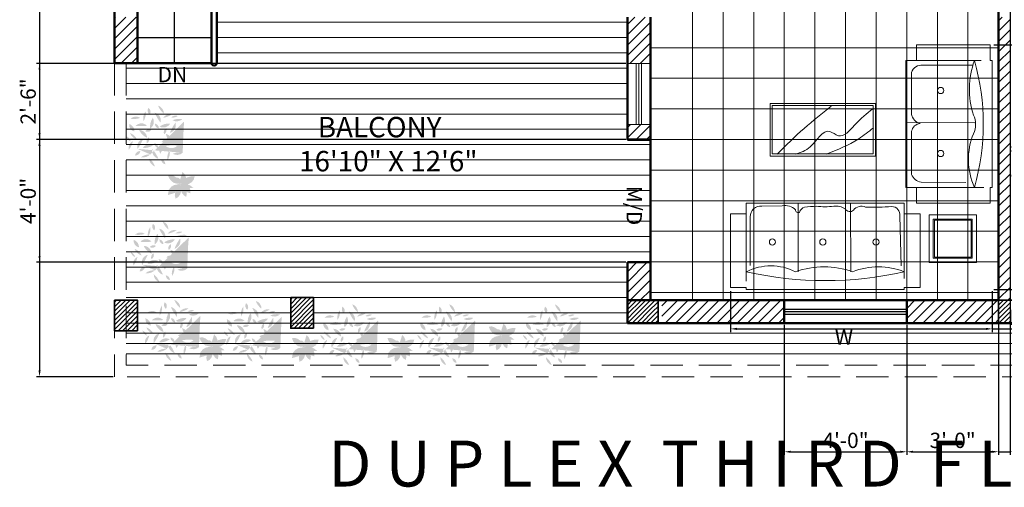
# Model space of a CAD drawing. Units: millimetres. Extents: x 225995 to 227247, y 225507 to 226008.
# Tile 11 of 23: x 226643 to 227029, y 225507 to 225691. Entities that reach past the tile are written whole.
import ezdxf

# ---------------------------------------------------------------- set-up
doc = ezdxf.new("R2010")
doc.units = ezdxf.units.MM
doc.linetypes.add('DASHED', pattern=[19.049999999999997, 12.7, -6.349999999999999])
for name, color, linetype, lineweight in [('A-ANNO-DIMS', 2, 'Continuous', 18), ('A-ANNO-TEXT', 3, 'Continuous', 18), ('A-AREA-IDEN', 30, 'Continuous', 18), ('A-COLS', 40, 'Continuous', 35), ('A-FLOR-PATT', 8, 'Continuous', 13), ('A-FLOR-STRS', 141, 'Continuous', 25), ('A-FURN', 9, 'Continuous', 18), ('A-GLAZ', 4, 'Continuous', 25), ('A-WALL', 7, 'Continuous', 50), ('A-WALL-OVHD', 1, 'DASHED', 18), ('A-WALL-PATT', 8, 'Continuous', 13)]:
    doc.layers.add(name, color=color, linetype=linetype, lineweight=lineweight)
doc.styles.get("Standard").update_dxf_attribs({"font": 'arial.ttf'})
doc.dimstyles.new('ISO-25', dxfattribs={"dimtxt": 6, "dimasz": 2.5, "dimexe": 1.25, "dimexo": 0.625, "dimtad": 1, "dimdec": 0, "dimlunit": 3, "dimtxsty": 'Standard', "dimcen": 2.5, "dimadec": 0, "dimazin": 0, "dimtfac": 1, "dimtdec": 0, "dimtmove": 0, "dimatfit": 3, "dimfxl": 1, "dimarcsym": 0})
pattern_1 = [(45, (646.0462645871739, 0.9310331261949613), (-2.020557627240559, 2.020557627240559), [])]
pattern_2 = [(45, (646.0462645871739, -119.068966873805), (-0.8980256121069157, 0.8980256121069157), [])]
pattern_3 = [(45, (500.5462645871448, -119.0689668737759), (-0.8980256121069157, 0.8980256121069157), [])]
pattern_4 = [(45, (0, 0), (-2.020557627240559, 2.020557627240559), [])]

# ---------------------------------------------------------------- blocks, each defined once
blk = doc.blocks.new('A$C412119AE')
for p, q in [((1765.943953579699, 2175.983816529711), (1765.943953579699, 2325.983816529712)), ((1765.943953579699, 2325.983816529712), (2465.943953579699, 2325.983816529712)), ((2465.943953579699, 2325.983816529712), (2465.943953579699, 2175.983816529711)), ((1665.943953579699, 2175.983816529711), (1765.943953579699, 2175.983816529711)), ((1665.943953579699, 2175.983816529711), (1665.943953579699, 970.8113427770732)), ((2379.086550219509, 2175.983816529711), (1665.943953579699, 2175.983816529711)), ((2465.943953579699, 2175.983816529711), (2485.943953579699, 2175.983816529711)), ((2485.943953579699, 2175.983816529711), (2485.943953579699, 970.8113427770732)), ((1719.402132396004, 1668.149708631943), (1719.402132396004, 2061.314478561108)), ((1825.749753817625, 2132.213049901882), (2302.702842007711, 2132.213049901882)), ((1375.364594020066, 1768.909058744728), (375.3645940200659, 1768.909058744728)), ((375.3645940200659, 1768.909058744728), (375.3645940200659, 1268.909058744728)), ((1355.364594020066, 1748.909058744757), (395.3645940200658, 1748.909058744728)), ((395.3645940200658, 1748.909058744728), (395.3645940200658, 1288.909058744728)), ((1355.364594020066, 1288.909058744728), (1355.364594020066, 1748.909058744757)), ((1375.364594020066, 1268.909058744728), (1375.364594020066, 1768.909058744728)), ((1669.166570326604, 1587.565689788869), (2319.166570326604, 1585.684169426706)), ((1719.402132396004, 1094.515882795851), (1719.402132396004, 1503.793962654425)), ((375.3645940200659, 1268.909058744728), (1375.364594020066, 1268.909058744728)), ((395.3645940200658, 1288.909058744728), (1355.364594020066, 1288.909058744728)), ((1665.943953579699, 970.8113427770732), (2404.343573573831, 970.8113427770732)), ((1765.943953579699, 820.8113427770732), (1765.943953579699, 970.8113427770732)), ((2235.027022214373, 1017.171979832055), (1809.636469750374, 1020.394664771796)), ((2485.943953579699, 970.8113427770732), (2465.943953579699, 970.8113427770732)), ((2465.943953579699, 970.8113427770732), (2465.943953579699, 820.8113427770732)), ((150.0000263674883, 819.9999771903385), (150.0000263674883, 81.60035719620646)), ((1650.000026367488, 819.9999771903385), (150.0000263674883, 819.9999771903385)), ((490.8466365284403, 797.2161591663316), (296.6958283240092, 793.0066807766561)), ((642.7067689166287, 819.9999771903385), (640.8252485544652, 169.9999771903385)), ((1139.574553680431, 819.9999771903385), (1143.479939016164, 169.9999771903385)), ((1650.000026367488, 106.8573805505293), (1650.000026367488, 819.9999771903385)), ((1650.000026367488, 819.9999771903385), (1650.000026367488, 719.9999771903385)), ((2465.943953579699, 820.8113427770732), (1765.943953579699, 820.8113427770732)), ((2.63674883172e-05, 19.99997719033854), (2.63674883172e-05, 719.9999771903385)), ((2.63674883172e-05, 719.9999771903385), (150.0000263674883, 719.9999771903385)), ((187.2489073937759, 691.9785491054063), (187.2489073937759, 228.9330189323518)), ((1620.533532246249, 224.7235405426764), (1607.905082460987, 700.3975441388028)), ((1650.000026367488, 719.9999771903385), (1800.000026367488, 719.9999771903385)), ((1800.000026367488, 719.9999771903385), (1800.000026367488, 19.99997719033854)), ((1885.77057496499, 708.9090587447572), (1885.77057496499, 258.9090587447572)), ((2335.770574964991, 708.9090587447572), (1885.77057496499, 708.9090587447572)), ((1925.77057496499, 668.9090587447572), (1925.77057496499, 298.9090587447572)), ((2295.77057496499, 668.9090587447572), (1925.77057496499, 668.9090587447572)), ((1935.77057496499, 658.9090587447572), (1935.77057496499, 308.9090587447572)), ((2285.770574964991, 658.909058744728), (1935.77057496499, 658.9090587447572)), ((2285.770574964991, 308.9090587447281), (2285.770574964991, 658.909058744728)), ((2295.77057496499, 298.9090587447281), (2295.77057496499, 668.9090587447572)), ((2335.770574964991, 258.9090587447572), (2335.770574964991, 708.9090587447572)), ((1925.77057496499, 298.9090587447572), (2295.77057496499, 298.9090587447281)), ((1935.77057496499, 308.9090587447572), (2285.770574964991, 308.9090587447281)), ((1885.77057496499, 258.9090587447572), (2335.770574964991, 258.9090587447572)), ((150.0000263674883, 19.99997719033854), (2.63674883172e-05, 19.99997719033854)), ((150.0000263674883, -2.28096614592e-05), (150.0000263674883, 19.99997719033854)), ((1650.000026367488, 19.99997719033854), (1650.000026367488, -2.28096614592e-05)), ((1800.000026367488, 19.99997719033854), (1650.000026367488, 19.99997719033854)), ((1650.000026367488, -2.28096614592e-05), (150.0000263674883, -2.28096614592e-05))]:
    blk.add_line(p, q)
for centre in [(1995.235273378755, 1891.710132711567), (1995.235273378755, 1293.146315121295), (398.2137806876563, 452.0367889854533), (876.4822162850469, 452.0367889854533), (1381.839690735214, 452.0367889854533)]:
    blk.add_circle(centre, 29.46649412123952)
for centre, radius, start, end in [((3089.318045017309, 1902.163791755767), 820.4175103410133, 160.5030351339521, 197.2788258837681), ((202.9249977454601, 1573.397579653392), 2197.261768790327, 344.0830231117248, 15.91697688827521), ((1812.799503640912, 2036.428557089559), 96.65597779210518, 82.30018877508738, 165.0800634395203), ((1830.015199570451, 1685.826864377537), 112.0166615508406, 189.0797032927071, 254.4408095684438), ((2133.531708251889, 1569.85852571376), 193.8393087278023, 332.7934666372156, 27.20653336278442), ((1809.099496729381, 1487.14361519317), 91.229662056465, 95.74420610428702, 169.4839915827727), ((2917.352403809986, 1237.925971360149), 658.0595328778988, 158.3005649339758, 203.9483253951991), ((1824.228147024347, 1130.144151438959), 110.7152512952639, 198.7718713191169, 262.4266896702824), ((284.8796445847838, 696.0098259844526), 97.71392959931639, 83.05443514735477, 182.3644604637284), ((515.9552177713776, 656.277232477616), 143.1580312389093, 45.31904974571957, 100.101392761676), ((643.8381095884251, 758.4502709400839), 27.22282178733356, 180.805938289541, 295.1831948509136), ((721.1300894821761, 716.6115292558679), 67.9230184061552, 104.6716568581485, 165.32843516604), ((1108.941975229507, -2844.008239933581), 3648.875507191725, 94.6209247707708, 96.37280966374853), ((897.5769615406753, 1374.681438045314), 587.5101224174774, 261.9179023631295, 278.0820976368704), ((996.1119805646013, 612.2990891316439), 181.4088900353399, 58.97104398562267, 95.03964304861204), ((1132.958847838919, 788.7824288163683), 48.17023342628601, 205.8893768857179, 315.6692558978528), ((1244.114162995305, 695.8341106949956), 96.94109095896602, 66.28266376022583, 142.2963408701175), ((1373.069186809036, 2811.282720742951), 2028.69077126019, 267.4583676811772, 274.482485251239), ((1532.549344049126, 712.4839583230786), 76.31886214712327, 350.8878572767813, 90.6975767837586), ((383.4446686404408, -290.5194572304899), 516.3085806814033, 63.11882319491773, 116.8811768050822), ((888.1632708451361, -595.1586895005894), 811.8234700655617, 70.47890614007272, 109.5210938599273), ((1404.718628572154, -452.9882930537278), 669.5351738080216, 68.50957107404854, 111.4904289259514), ((900.0000263674882, 3466.442302512354), 3380.685138278112, 257.1823712023422, 282.8176287976578)]:
    blk.add_arc(centre, radius, start, end)
for points, knots in [([(954.7218874091631, 1741.2770716144), (867.8962163294796, 1672.869149598936), (688.1710409575262, 1531.267873983376), (525.7976649372246, 1370.039222415447), (441.8672633597598, 1286.700526112196)], [0, 0, 0, 0, 331.319965476721, 685.8172031274577, 685.8172031274577, 685.8172031274577, 685.8172031274577]), ([(1351.018605932317, 1717.965428392053), (1294.335371423013, 1672.145785582451), (1194.024907101795, 1591.06026382188), (1053.454737117002, 1416.247750486856), (895.9202696333112, 1563.202916472364), (786.5878530944017, 1342.910342559372), (665.0576220379807, 1302.69937452165), (616.7040548715886, 1286.700526112196)], [0, 0, 0, 0, 235.2190389939173, 416.2594323158832, 507.4804419009926, 744.1389804191335, 900.5178576378909, 900.5178576378909, 900.5178576378909, 900.5178576378909]), ([(1356.846481175365, 1537.300422957429), (1311.253733790716, 1500.622310124164), (1176.602655951446, 1392.299216882096), (1014.989694033541, 1328.739183180236), (908.098751909667, 1286.700526112196)], [0, 0, 0, 0, 174.8368930376187, 516.3535308580789, 516.3535308580789, 516.3535308580789, 516.3535308580789])]:
    blk.add_open_spline(points, degree=3, knots=knots)
blk = doc.blocks.new('A$C24925061')
h = blk.add_hatch(color=256)
edge = h.paths.add_edge_path()
edge.add_arc((0.9654668007644887, -0.4430118219963788), 1.340452708384529, 19.29877617203986, 52.5009711306829)
edge.add_arc((2.430682118670802, 0.6176222582514584), 0.6492236151388806, 179.7500334610202, 252.0497138534684)
edge = h.paths.add_edge_path()
edge.add_arc((1.054811990629332, 0.8270366531730815), 0.3581084080100917, 82.8639188084402, 178.5781836737518)
edge.add_arc((0.6842907764571465, 1.257487300113325), 0.4217509294388061, 271.7015353359617, 349.7405671458981)
edge = h.paths.add_edge_path()
edge.add_arc((0.7398896939064344, 3.208054826131274), 0.5131669839777279, 170.7089921054556, 259.1064421702567)
edge.add_arc((0.0380644111778565, 2.718314181925279), 0.6050105769437998, 358.6570906337592, 431.1583436420608)
edge = h.paths.add_edge_path(flags=17)
edge.add_arc((3.592640665857516, -1.494224689759221), 3.12619905091911, 83.18118726980056, 99.80780028268723)
edge.add_arc((3.499851110983627, 2.06232682614268), 0.6480638406530903, 227.2701766889413, 315.7188108934203)
edge = h.paths.add_edge_path()
edge.add_arc((3.734261480343548, 5.152744740282059), 1.340452708384864, 199.2987761720417, 232.5009711306753)
edge.add_arc((2.269046162456106, 4.092110659996023), 0.6492236151388806, 359.7500334610202, 432.0497138534683)
edge = h.paths.add_edge_path()
edge.add_arc((4.227760104328808, 0.6480348606876305), 1.049859166199157, 145.1988769454638, 189.1497824077265)
edge.add_arc((2.410856579678011, 1.061681349184937), 0.9726839997093691, 323.3521143936382, 370.9965449625487)
edge = h.paths.add_edge_path()
edge.add_arc((-0.3783952598837459, -0.636052571697519), 3.126199029022735, 23.1811872412288, 39.80780036797759)
edge.add_arc((2.655273905518924, 1.222581287542425), 0.6480638406530903, 167.2701766887328, 255.7188108934403)
edge = h.paths.add_edge_path()
edge.add_arc((2.679624522240374, 0.187533518554801), 0.3505395552648481, 356.5426824596368, 444.4722527015056)
edge.add_arc((3.095116252619618, 0.5424906454215943), 0.3817729323924592, 180.9076653059353, 260.1072698550584)
edge = h.paths.add_edge_path()
edge.add_arc((-0.2543802208936086, 1.774411871719848), 0.6256841278847063, 16.02384347117297, 66.01086962640353)
edge.add_arc((0.5364094056467366, 2.462255490477446), 0.5488520080281845, 192.2233289830762, 249.8113841143446)
edge = h.paths.add_edge_path()
edge.add_arc((2.085901736917776, 4.330812086120431), 0.4217509294388061, 151.7015353360343, 229.7405671459502)
edge.add_arc((1.527859934137268, 4.225156625798945), 0.3581084080100917, 322.863918808216, 418.5781836737615)
edge = h.paths.add_edge_path()
edge.add_arc((2.604326971678574, 5.421898561365878), 1.678331187938795, 278.1970065494975, 305.0866342104797)
edge.add_arc((3.433432828821423, 3.332273650905108), 0.7290003658907461, 79.2782419008663, 144.0053988714987)
edge = h.paths.add_edge_path()
edge.add_arc((1.244192236909384, 1.665355477786988), 0.9726839997093691, 263.3521143934827, 310.9965449624541)
edge.add_arc((1.767437406342878, -0.0649826458809457), 0.9941318350168211, 82.61547307824048, 129.7622598979537)
edge.add_arc((5.655552472019962, 2.47369755367049), 1.54277222239035, 140.3878455158555, 169.0632147292559)
edge.add_arc((3.867947864109055, 3.318035527745678), 0.6150719187256568, 296.2514800948445, 373.0911385647991)
edge.add_arc((4.121129142004292, -0.2555835587211277), 1.336065046305859, 79.27146673985777, 112.5691371544225)
edge.add_arc((3.935011726609218, 1.539217413818505), 0.6492236151388806, 239.7500334609024, 312.0497138533913)
edge.add_arc((-2.105002859595515, 3.543752988587357), 3.700911033329421, 323.811293257942, 337.500285939478)
edge.add_arc((1.457511089847002, 1.539538388494975), 0.6033752219542029, 103.823213301674, 197.4539371695969)
h = blk.add_hatch(color=256)
h.paths.add_polyline_path([(2.851168543304311, 1.818131605252574, 0.3946244384457369), (2.636548992306188, 0.985638457603045, 0.1798480615289245)])
h.paths.add_polyline_path([(3.082036725636953, 2.529751717409226, 0.394624438535923), (3.695687164500213, 1.927639160092212, 0.179848061560959)])
h.paths.add_polyline_path([(3.231407417620403, 2.01596347390091, 0.4036687984612434), (2.752868403749062, 1.927206996393806, 0.3600202040609362)])
h.paths.add_polyline_path([(1.004955914334459, 2.820119584196845, 0.1798480615609561), (1.618606353197719, 2.218007026879831, 0.3946244385359146)])
h.paths.add_polyline_path([(0.7368288115003452, 3.137897310306243, 0.0598006304704098), (1.618883747633844, 3.147993476542751, 0.4314732228430921)])
h.paths.add_polyline_path([(0.2906494142400788, 2.592000309059812, 0.2079726492074865), (0.8565059954883054, 2.061536986476085, 0.2022718347148865)])
h.paths.add_polyline_path([(0.5255993990563184, 1.969866162593234, 0.351061284593648), (0.2002188232393109, 1.28329626122354, 0.1250427165750839)])
h.paths.add_polyline_path([(2.064094086547356, 3.762120286686013, 0.179848061528906), (1.849474535530362, 2.929627139036028, 0.3946244384456845)])
h.paths.add_polyline_path([(2.205234118591988, 4.153214032784262, 0.0598006305081244), (2.655005123326645, 3.394380133124059, 0.4314732235157507)])
h.paths.add_polyline_path([(4.000755981485554, 3.901763793001691, 0.2567008059800083), (3.481778020596721, 3.800721533467594, 0.2216352721376879)])
h = blk.add_hatch(color=256)
edge = h.paths.add_edge_path()
edge.add_arc((4.783666011938521, 3.136866607786714), 1.049859166456769, 205.198876949193, 249.1497824052312)
edge.add_arc((3.516985882185736, 1.770205243277587), 0.9726839997093691, 23.35211439366051, 70.99654496241732)
edge = h.paths.add_edge_path()
edge.add_arc((6.321357472290628, 1.515707272357531), 3.126199036238745, 143.181187250639, 159.8078003422576)
edge.add_arc((3.194898744882266, 3.213624910442149), 0.6480638406530903, 287.2701766888658, 375.7188108934812)
edge = h.paths.add_edge_path()
edge.add_arc((3.91039601142279, 4.138007997924205), 0.6492236151388806, 239.7500334609024, 312.0497138533913)
edge.add_arc((4.09632440989958, 2.338777269955016), 1.34045270878445, 79.29877617472617, 112.5009711135879)
edge = h.paths.add_edge_path()
edge.add_arc((2.569644433533767, 3.294740799551846), 0.3505395552648481, 176.5426824596367, 264.4722527015058)
edge.add_arc((2.154152703684076, 2.939783673252577), 0.3817729323924592, 0.9076653059353086, 80.1072698550584)
edge = h.paths.add_edge_path()
edge.add_arc((0.5884063799751403, 5.211744072890041), 1.54277222239035, 260.3878455157838, 289.0632147295259)
edge.add_arc((0.7513421283861135, 3.240673488840684), 0.6158895154720025, 56.38628213043215, 133.0647780659807)
edge = h.paths.add_edge_path()
edge.add_arc((0.4728829745058647, 4.099723883600972), 1.049859166198971, 325.1988769454567, 369.1497824077285)
edge.add_arc((2.289786499156662, 3.686077395104121), 0.9726839997093691, 143.3521143936382, 190.9965449625486)
edge = h.paths.add_edge_path()
edge.add_arc((1.828539176611457, 1.104062448752529), 0.629455908225403, 62.47292702239469, 148.6145416403691)
edge.add_arc((1.395433377251947, 2.661175117739958), 1.233708969597487, 265.1526518033275, 305.9348168593484)
edge = h.paths.add_edge_path()
edge.add_arc((5.655552472019962, 2.47369755367049), 1.54277222239035, 140.3878455158555, 169.0632147292559)
edge.add_arc((3.867947864109055, 3.318035527745678), 0.6150719187256568, 296.2514800948445, 373.0911385647991)
h = blk.add_hatch(color=256)
h.paths.add_polyline_path([(4.369845577160731, 1.057127354919202, 0.146319487598694), (3.608350086608197, 0.9781617343940069, 0.3261687141928539)])
h.paths.add_polyline_path([(1.873287995879991, 0.9234978840620442, 0.2028818153507969), (1.131587204366269, 0.6992114564484382, 0.2077538311609659)])
h.paths.add_polyline_path([(1.313348523569629, 2.125438391000216, 0.4328978137907586), (0.8819162319473434, 1.358562649704026, 0.0596498710153214)])
h.paths.add_polyline_path([(4.467034684897271, 3.457349727895916, 0.1257036487768282), (4.140885987354067, 2.766838424998468, 0.3479812378174587)])
h = blk.add_hatch(color=256)
edge = h.paths.add_edge_path()
edge.add_arc((2.872103902223216, 3.643696295536074), 0.629455908225403, 242.4729270223947, 328.6145416403691)
edge.add_arc((3.305209701582725, 2.086583626510901), 1.233708969597487, 85.15265180332744, 125.9348168593483)
edge = h.paths.add_edge_path()
edge.add_arc((1.662493596921649, 3.024249284020925), 0.3505395552648481, 236.5426824596533, 324.4722527014114)
edge.add_arc((1.762149620581567, 2.486944327342598), 0.3817729323924592, 60.90766530602383, 140.1072698549302)
edge = h.paths.add_edge_path()
edge.add_arc((1.443170702256793, 2.103387856310973), 0.3505395552648481, 296.5426824596887, 384.4722527013205)
edge.add_arc((1.958318456314827, 1.92104002649944), 0.3817729323924592, 120.9076653060203, 200.1072698549525)
edge = h.paths.add_edge_path()
edge.add_arc((3.257472376577879, 2.644370887939885), 0.3505395552648481, 116.5426824596887, 204.4722527013206)
edge.add_arc((2.742324622538717, 2.826718717789617), 0.3817729323924592, 300.9076653060203, 380.1072698549526)
edge = h.paths.add_edge_path()
edge.add_arc((2.130998645320005, 1.453017944169687), 0.3505395552648481, 356.5426824596368, 444.4722527015056)
edge.add_arc((2.546490375150597, 1.80797507103648), 0.3817729323924592, 180.9076653059353, 260.1072698550584)
blk = doc.blocks.new('A$C5FD41495')
h = blk.add_hatch(color=256)
h.paths.add_polyline_path([(1.005244618128244, 1.65167951100625), (1.161399103884377, 1.821900903511277), (1.282585341968342, 1.865935267084068), (1.285418139069633, 1.875219105078713), (0.8140981972906047, 1.781604425842715), (0.4284727904075681, 1.547567727812065), (0.128541918360952, 1.173109010926737), (1.160472038e-07, 0.4709989167160984), (0.9426399996048075, 0.7518429544240917), (0.9448716245508421, 0.7591566012094974), (0.953351816452141, 0.8425321748748046), (1.041205084484772, 1.098459985348426), (0.8881287537963088, 1.098459985348426), (0.8881287537963088, 1.396347422218468)])
h.paths.add_polyline_path([(1.12236048246018, 2.460231125392283), (1.12236048246018, 2.754156926702535), (1.11402906933722, 2.76455855770223), (0.7712509298723944, 2.998595255733334), (0.3856255229595717, 3.139017274587104), (1.160472038e-07, 3.092209934968423), (0.1713891857793897, 2.670943878465777), (0.4284727904075681, 2.34329250119913), (0.7712509298723944, 2.062448463550254), (1.199723604203427, 1.968833784313801), (1.43835878248069, 1.968833784313801), (1.395630832518463, 1.992122296016759), (1.239476346762558, 2.204899036604501)])
h.paths.add_polyline_path([(3.38493424336525, 2.483714519993782), (3.51347604564944, 2.904980576555999), (2.999308836452428, 2.904980576555999), (2.485141627225857, 2.76455855770223), (2.356599824941213, 2.687964723925006), (2.356599824941213, 2.436907180435127), (1.707939804060742, 2.161336191816872), (1.707939804060742, 2.119788340381774), (1.668739779550833, 1.991594467696131), (1.726823075758602, 1.942243278054093), (1.864094289816875, 1.992122296016759), (1.868892411952629, 1.991375102766369), (1.928127150580621, 2.015641123932482), (2.270905290075006, 1.968833784313801), (2.475253795472781, 1.857216276717963), (2.576957204885729, 1.881905861185941), (2.742225231824249, 1.922026444696484), (3.127850638737072, 2.156063142727589)])
h.paths.add_polyline_path([(2.859271422936217, 1.409428994351173), (2.827919766720015, 1.500760388193839), (2.61368342954006, 1.781604425842715), (2.475253795472781, 1.857216276717963), (2.270905290075006, 1.968833784313801), (1.928127150580621, 2.015641123932482), (1.868892411952629, 1.991375102766369), (2.137364639904944, 1.949566947875837), (2.371596368539258, 1.779345555370355), (2.527750854295391, 1.56656881472395), (2.605828097173343, 1.268681377853908), (2.293519125661077, 1.311236725994831), (2.020248775573008, 1.396347422218468), (1.786017046938468, 1.609124162865327), (1.644426488478984, 1.879228786130852, -0.1725597637911187), (1.643260679139302, 1.879063224815809), (1.62986256118279, 1.813199379104617), (1.62986256118279, 1.802277667499083), (1.842432615714415, 1.453953048575613), (2.142363487761031, 1.12630167130942), (2.461147157475124, 0.894137266822554), (2.527988894673853, 0.8454576336009721), (2.956461569004886, 0.7050356148058654), (2.956461569004886, 1.12630167130942)])
h.paths.add_polyline_path([(1.724602630277331, 0.8893395144925761), (1.736980734523967, 1.011038597487868), (1.7674498977251, 1.310605570996131), (1.638908095411125, 1.731871627498321), (1.62986256118279, 1.726225029886563), (1.62986256118279, 1.65167951100625), (1.551785318275051, 1.396347422218468), (1.356592211094266, 1.183570681631181), (1.161399103884377, 1.098459985348426), (1.048403985997538, 1.098459985348426), (0.9448716245508421, 0.7591566012094974), (0.9105045490334759, 0.4212661183717046), (0.9961990838999099, 6.18690592e-08), (1.338977223364508, 0.1872294203415095), (1.596060827992459, 0.5148807976077024)])
h = blk.add_hatch(color=256)
h.paths.add_polyline_path([(2.371596368539258, 1.779345555370355), (2.137364639904944, 1.949566947875837), (1.868892411952629, 1.991375102766369), (1.799585348295977, 1.96298286686283), (1.78122223062769, 1.955460260353675), (1.734023866023562, 1.93612503771169), (1.64767231114024, 1.90075037910924), (1.643961051527867, 1.882506187459284, -0.7056699890938171), (1.644426488478984, 1.879228786130852), (1.786017046938468, 1.609124162865327), (2.020248775573008, 1.396347422218468), (2.293519125661077, 1.311236725994831), (2.605828097173343, 1.268681377853908), (2.527750854295391, 1.56656881472395)])
h.paths.add_polyline_path([(1.62986256118279, 1.65167951100625), (1.62986256118279, 1.726225029886563), (1.609596665373373, 1.713574217205632), (1.62819627853446, 1.805008095651146), (1.62986256118279, 1.813199379104617), (1.62986256118279, 1.864456251653109), (1.551785318304382, 1.907011599734914), (1.395630832518463, 1.907011599734914), (1.161399103884377, 1.821900903511277), (1.005244618128244, 1.65167951100625), (0.8881287537963088, 1.396347422218468), (0.8881287537963088, 1.098459985348426), (1.161399103884377, 1.098459985348426), (1.356592211094266, 1.183570681631181), (1.551785318275051, 1.396347422277585)])
h.paths.add_polyline_path([(1.707939804060742, 2.375120429110438), (1.551785318275051, 2.587897169755933), (1.356592211094266, 2.75811856226187), (1.12236048246018, 2.75811856226187), (1.12236048246018, 2.460231125392283), (1.239476346762558, 2.204899036604501), (1.395630832518463, 1.992122296016759), (1.551785318275051, 1.907011599734914), (1.62986256118279, 1.907011599734914), (1.644502044212913, 1.912331018251961), (1.707939804060742, 2.119788340381774)])
h = blk.add_hatch(color=256)
h.paths.add_polyline_path([(2.91361430155689, 1.734797086224489), (2.576957204885729, 1.881905861185941), (2.475253795472781, 1.857216276717963), (2.61368342954006, 1.781604425842715), (2.827919766720015, 1.500760388193839), (2.859271422936217, 1.409428994351173), (2.870767034138452, 1.407145708957841), (3.342086975917254, 1.407145708957841)])
h.paths.add_polyline_path([(2.461147157475124, 0.894137266822554), (2.142363487761031, 1.12630167130942), (1.842432615714415, 1.453953048575613), (1.62986256118279, 1.802277667499083), (1.62986256118279, 1.726225029886563), (1.638908095411125, 1.731871627498321), (1.7674498977251, 1.310605570996131), (1.736980734523967, 1.011038597487868), (1.842432615714415, 0.7518429544240917), (2.09951622034282, 0.4241915770983269), (2.39944709235965, 0.236962218684539), (2.485141627225857, 0.6582282751880939)])
h.paths.add_polyline_path([(2.356599824941213, 2.687964723925006), (2.356599824941213, 2.858173236938682), (2.185210755179014, 3.232631953823101), (1.928127150580621, 3.513475991471977), (1.608721980542668, 2.51031504102616), (1.707939804060742, 2.375120429110438), (1.707939804060742, 2.161336191816872), (2.356599824941213, 2.436907180435127)])
blk = doc.blocks.new('*D89')
at = {"layer": 'A-ANNO-DIMS', "color": 0, "lineweight": -2, "transparency": 16777216}
for p, q in [((226921.3437957988, 225584.2201883473), (226921.3437957988, 225568.2009671293)), ((227023.9719372525, 225584.2201883473), (227023.9719372525, 225568.2009671293)), ((226923.8437957988, 225569.4509671293), (227021.4719372525, 225569.4509671293)), ((227023.9719372525, 225569.4509671293), (227138.893833569, 225569.4509671293))]:
    blk.add_line(p, q, dxfattribs=at)
at = {"layer": 'A-ANNO-DIMS', "color": 0, "transparency": 16777216}
for points in [[(226923.8437957988, 225569.867633796), (226923.8437957988, 225569.0343004626), (226921.3437957988, 225569.4509671293)], [(227021.4719372525, 225569.867633796), (227021.4719372525, 225569.0343004626), (227023.9719372525, 225569.4509671293)]]:
    blk.add_solid(points, dxfattribs=at)
at = {"layer": 'Defpoints', "color": 0, "transparency": 16777216}
for p in [(226921.3437957988, 225584.8451883474), (227023.9719372525, 225584.8451883474), (227023.9719372525, 225569.4509671293)]:
    blk.add_point(p, dxfattribs=at)
at = {"layer": 'A-ANNO-DIMS', "color": 0, "transparency": 16777216, "insert": (227082.6828854108, 225573.18033275), "char_height": 6, "attachment_point": 5}
blk.add_mtext('LOUNGE SOFA SET 8\'-6 1/2"', dxfattribs=at)
blk = doc.blocks.new('*D90')
at = {"layer": 'A-ANNO-DIMS', "color": 0, "lineweight": -2, "transparency": 16777216}
for p, q in [((227024.5969372526, 225680.8696384044), (227040.6161584708, 225680.8696384044)), ((227039.3661584708, 225587.3451883475), (227039.3661584708, 225678.3696384044)), ((227024.5969372526, 225584.8451883474), (227040.6161584708, 225584.8451883474))]:
    blk.add_line(p, q, dxfattribs=at)
at = {"layer": 'A-ANNO-DIMS', "color": 0, "transparency": 16777216}
for points in [[(227038.9494918042, 225678.3696384044), (227039.7828251375, 225678.3696384044), (227039.3661584708, 225680.8696384044)], [(227038.9494918042, 225587.3451883475), (227039.7828251375, 225587.3451883475), (227039.3661584708, 225584.8451883474)]]:
    blk.add_solid(points, dxfattribs=at)
at = {"layer": 'Defpoints', "color": 0, "transparency": 16777216}
for p in [(227023.9719372526, 225680.8696384044), (227039.3661584708, 225680.8696384044), (227023.9719372526, 225584.8451883474)]:
    blk.add_point(p, dxfattribs=at)
at = {"layer": 'A-ANNO-DIMS', "color": 0, "transparency": 16777216, "insert": (227035.6777205445, 225632.8574133758), "char_height": 6, "attachment_point": 5, "rotation": 90}
blk.add_mtext('8\'-0"', dxfattribs=at)
blk = doc.blocks.new('*D113')
at = {"layer": 'A-ANNO-DIMS', "color": 0, "lineweight": -2, "transparency": 16777216}
for p, q in [((226679.2976550001, 225961.7046240002), (226649.2226550003, 225961.7046240002)), ((226650.4726550003, 225959.2046240001), (226650.4726550003, 225553.2046240001)), ((226679.2976550001, 225550.7046240001), (226649.2226550003, 225550.7046240001))]:
    blk.add_line(p, q, dxfattribs=at)
at = {"layer": 'A-ANNO-DIMS', "color": 0, "transparency": 16777216}
for points in [[(226650.0559883336, 225959.2046240001), (226650.8893216669, 225959.2046240001), (226650.4726550003, 225961.7046240002)], [(226650.0559883336, 225553.2046240001), (226650.8893216669, 225553.2046240001), (226650.4726550003, 225550.7046240001)]]:
    blk.add_solid(points, dxfattribs=at)
at = {"layer": 'Defpoints', "color": 0, "transparency": 16777216}
for p in [(226679.9226550001, 225961.7046240002), (226650.4726550003, 225550.7046240001), (226679.9226550001, 225550.7046240001)]:
    blk.add_point(p, dxfattribs=at)
at = {"layer": 'A-ANNO-DIMS', "color": 0, "transparency": 16777216, "insert": (226646.7821706892, 225756.204624), "char_height": 6, "attachment_point": 5, "rotation": 90}
blk.add_mtext('34\'-3"', dxfattribs=at)
blk = doc.blocks.new('*D115')
at = {"layer": 'A-ANNO-DIMS', "color": 0, "lineweight": -2, "transparency": 16777216}
for p, q in [((227026.422655, 225740.579624), (227026.422655, 225520.004624)), ((227030.922655, 225740.579624), (227030.922655, 225520.004624)), ((227023.922655, 225521.254624), (227021.422655, 225521.254624)), ((227026.422655, 225521.254624), (227030.922655, 225521.254624)), ((227033.422655, 225521.254624), (227067.1030779195, 225521.254624))]:
    blk.add_line(p, q, dxfattribs=at)
at = {"layer": 'A-ANNO-DIMS', "color": 0, "transparency": 16777216}
for points in [[(227023.922655, 225521.6712906667), (227023.922655, 225520.8379573334), (227026.422655, 225521.254624)], [(227033.422655, 225521.6712906667), (227033.422655, 225520.8379573334), (227030.922655, 225521.254624)]]:
    blk.add_solid(points, dxfattribs=at)
at = {"layer": 'Defpoints', "color": 0, "transparency": 16777216}
for p in [(227026.422655, 225741.204624), (227030.922655, 225741.204624), (227030.922655, 225521.254624)]:
    blk.add_point(p, dxfattribs=at)
at = {"layer": 'A-ANNO-DIMS', "color": 0, "transparency": 16777216, "insert": (227051.5128664598, 225524.9819432361), "char_height": 6, "attachment_point": 5}
blk.add_mtext('0\'-4 1/2"', dxfattribs=at)
blk = doc.blocks.new('*D131')
at = {"layer": 'A-ANNO-DIMS', "color": 0, "lineweight": -2, "transparency": 16777216}
for p, q in [((226942.422655, 225571.079624), (226942.422655, 225520.004624)), ((226990.422655, 225571.079624), (226990.422655, 225520.004624)), ((226944.922655, 225521.254624), (226987.922655, 225521.254624))]:
    blk.add_line(p, q, dxfattribs=at)
at = {"layer": 'A-ANNO-DIMS', "color": 0, "transparency": 16777216}
for points in [[(226944.922655, 225521.6712906667), (226944.922655, 225520.8379573334), (226942.422655, 225521.254624)], [(226987.922655, 225521.6712906667), (226987.922655, 225520.8379573334), (226990.422655, 225521.254624)]]:
    blk.add_solid(points, dxfattribs=at)
at = {"layer": 'Defpoints', "color": 0, "transparency": 16777216}
for p in [(226942.422655, 225571.704624), (226990.422655, 225571.704624), (226990.422655, 225521.254624)]:
    blk.add_point(p, dxfattribs=at)
at = {"layer": 'A-ANNO-DIMS', "color": 0, "transparency": 16777216, "insert": (226966.422655, 225524.9430619263), "char_height": 6, "attachment_point": 5}
blk.add_mtext('4\'-0"', dxfattribs=at)
blk = doc.blocks.new('*D132')
at = {"layer": 'A-ANNO-DIMS', "color": 0, "lineweight": -2, "transparency": 16777216}
for p, q in [((226990.422655, 225571.079624), (226990.422655, 225520.004624)), ((227026.422655, 225571.079624), (227026.422655, 225520.004624)), ((226992.922655, 225521.254624), (227023.922655, 225521.254624))]:
    blk.add_line(p, q, dxfattribs=at)
at = {"layer": 'A-ANNO-DIMS', "color": 0, "transparency": 16777216}
for points in [[(226992.922655, 225521.6712906667), (226992.922655, 225520.8379573334), (226990.422655, 225521.254624)], [(227023.922655, 225521.6712906667), (227023.922655, 225520.8379573334), (227026.422655, 225521.254624)]]:
    blk.add_solid(points, dxfattribs=at)
at = {"layer": 'Defpoints', "color": 0, "transparency": 16777216}
for p in [(226990.422655, 225571.704624), (227026.422655, 225571.704624), (227026.422655, 225521.254624)]:
    blk.add_point(p, dxfattribs=at)
at = {"layer": 'A-ANNO-DIMS', "color": 0, "transparency": 16777216, "insert": (227008.422655, 225524.9451083111), "char_height": 6, "attachment_point": 5}
blk.add_mtext('3\'-0"', dxfattribs=at)
blk = doc.blocks.new('*D133')
at = {"layer": 'A-ANNO-DIMS', "color": 0, "lineweight": -2, "transparency": 16777216}
for p, q in [((226880.2976550001, 225673.5601360001), (226649.2226550003, 225673.5601360001)), ((226650.4726550003, 225671.0601360001), (226650.4726550003, 225646.2046240002)), ((226880.2976550001, 225643.7046240002), (226649.2226550003, 225643.7046240002))]:
    blk.add_line(p, q, dxfattribs=at)
at = {"layer": 'A-ANNO-DIMS', "color": 0, "transparency": 16777216}
for points in [[(226650.0559883336, 225671.0601360001), (226650.8893216669, 225671.0601360001), (226650.4726550003, 225673.5601360001)], [(226650.0559883336, 225646.2046240002), (226650.8893216669, 225646.2046240002), (226650.4726550003, 225643.7046240002)]]:
    blk.add_solid(points, dxfattribs=at)
at = {"layer": 'Defpoints', "color": 0, "transparency": 16777216}
for p in [(226880.9226550001, 225673.5601360001), (226650.4726550003, 225643.7046240002), (226880.9226550001, 225643.7046240002)]:
    blk.add_point(p, dxfattribs=at)
at = {"layer": 'A-ANNO-DIMS', "color": 0, "transparency": 16777216, "insert": (226646.7842170739, 225658.63238), "char_height": 6, "attachment_point": 5, "rotation": 90}
blk.add_mtext('2\'-6"', dxfattribs=at)
blk = doc.blocks.new('*D134')
at = {"layer": 'A-ANNO-DIMS', "color": 0, "lineweight": -2, "transparency": 16777216}
for p, q in [((226880.2976550001, 225643.7046240002), (226649.2226550003, 225643.7046240002)), ((226650.4726550003, 225641.2046240001), (226650.4726550003, 225598.0601360001)), ((226880.2976550001, 225595.5601360001), (226649.2226550003, 225595.5601360001))]:
    blk.add_line(p, q, dxfattribs=at)
at = {"layer": 'A-ANNO-DIMS', "color": 0, "transparency": 16777216}
for points in [[(226650.0559883336, 225641.2046240001), (226650.8893216669, 225641.2046240001), (226650.4726550003, 225643.7046240002)], [(226650.0559883336, 225598.0601360001), (226650.8893216669, 225598.0601360001), (226650.4726550003, 225595.5601360001)]]:
    blk.add_solid(points, dxfattribs=at)
at = {"layer": 'Defpoints', "color": 0, "transparency": 16777216}
for p in [(226880.9226550001, 225643.7046240002), (226650.4726550003, 225595.5601360001), (226880.9226550001, 225595.5601360001)]:
    blk.add_point(p, dxfattribs=at)
at = {"layer": 'A-ANNO-DIMS', "color": 0, "transparency": 16777216, "insert": (226646.7842170739, 225619.63238), "char_height": 6, "attachment_point": 5, "rotation": 90}
blk.add_mtext('4\'-0"', dxfattribs=at)

msp = doc.modelspace()

# ---------------------------------------------------------------- hatches: boundary and pattern name
at = {"layer": 'A-WALL-PATT'}
h = msp.add_hatch(dxfattribs=at)
h.set_pattern_fill('ANSI31', color=256, scale=0.9)
h.set_pattern_definition(pattern_1)
h.paths.add_polyline_path([(226688.9226552027, 225691.7046236642), (226679.9226552027, 225691.7046236642), (226679.9226552027, 225673.7046236642), (226688.9226552027, 225673.7046236642)])
h = msp.add_hatch(dxfattribs=at)
h.set_pattern_fill('ANSI31', color=256, scale=0.9)
h.set_pattern_definition(pattern_4)
h.paths.add_polyline_path([(226889.9226552027, 225691.7046236642), (226882.4226552026, 225691.7046236642), (226880.9226552027, 225691.7046236642), (226880.9226552027, 225673.5601360966), (226889.9226552027, 225673.5601360966)])
h = msp.add_hatch(dxfattribs=at)
h.set_pattern_fill('ANSI31', color=256, scale=0.9)
h.set_pattern_definition(pattern_1)
h.paths.add_polyline_path([(227030.9226552027, 225691.7046236642), (227026.4226552027, 225691.7046236642), (227026.4226552027, 225580.7046236641), (227030.9226552027, 225580.7046236641)])
h = msp.add_hatch(dxfattribs=at)
h.set_pattern_fill('ANSI31', color=256, scale=0.9)
h.set_pattern_definition(pattern_4)
h.paths.add_polyline_path([(226889.9226552027, 225649.5601360966), (226880.9226552027, 225649.5601360966), (226880.9226552027, 225643.5601360966), (226889.9226552027, 225643.5601360966)])
h = msp.add_hatch(dxfattribs=at)
h.set_pattern_fill('ANSI31', color=256, scale=0.9)
h.set_pattern_definition(pattern_4)
h.paths.add_polyline_path([(226889.9226552027, 225595.5601360966), (226880.9226552027, 225595.5601360966), (226880.9226552027, 225580.7046236642), (226889.9226552027, 225580.7046236642)])
h = msp.add_hatch(dxfattribs=at)
h.set_pattern_fill('ANSI31', color=256, scale=0.4000000000000002)
h.set_pattern_definition([(45, (646.0462645871448, -1.068966873805038), (-0.8980256121069157, 0.8980256121069157), [])])
h.paths.add_polyline_path([(226757.9226552026, 225581.7046236642), (226748.9226552026, 225581.7046236642), (226748.9226552026, 225569.7046236642), (226757.9226552026, 225569.7046236642)])
h = msp.add_hatch(dxfattribs=at)
h.set_pattern_fill('ANSI31', color=256, scale=0.4000000000000002)
h.set_pattern_definition([(45, (577.0462645871739, -2.068966873834142), (-0.8980256121069157, 0.8980256121069157), [])])
h.paths.add_polyline_path([(226688.9226552026, 225580.7046236642), (226679.9226552026, 225580.7046236642), (226679.9226552026, 225568.7046236642), (226688.9226552026, 225568.7046236642)])
h = msp.add_hatch(dxfattribs=at)
h.set_pattern_fill('ANSI31', color=256, scale=0.4000000000000002)
h.set_pattern_definition(pattern_3)
h.paths.add_polyline_path([(226885.4226552026, 225580.7046236642), (226880.9226552026, 225580.7046236642), (226880.9226552026, 225576.2046236643), (226885.4226552026, 225576.2046236643)])
h = msp.add_hatch(dxfattribs=at)
h.set_pattern_fill('ANSI31', color=256, scale=0.4000000000000002)
h.set_pattern_definition(pattern_3)
h.paths.add_polyline_path([(226892.9226552026, 225580.7046236642), (226885.4226552026, 225580.7046236642), (226885.4226552026, 225576.2046236643), (226892.9226552026, 225576.2046236643)])
h = msp.add_hatch(dxfattribs=at)
h.set_pattern_fill('ANSI31', color=256, scale=0.9)
h.set_pattern_definition(pattern_1)
h.paths.add_polyline_path([(226942.4226552026, 225580.7046236642), (226894.4226552026, 225580.7046236642), (226894.4226552026, 225571.7046236642), (226942.4226552026, 225571.7046236642)])
h = msp.add_hatch(dxfattribs=at)
h.set_pattern_fill('ANSI31', color=256, scale=0.9)
h.set_pattern_definition(pattern_1)
h.paths.add_polyline_path([(227026.4226552027, 225580.7046236642), (226990.4226552026, 225580.7046236642), (226990.4226552026, 225571.7046236642), (227026.4226552027, 225571.7046236642)])
h = msp.add_hatch(dxfattribs=at)
h.set_pattern_fill('ANSI31', color=256, scale=0.4000000000000002)
h.set_pattern_definition(pattern_2)
h.paths.add_polyline_path([(227030.9226552027, 225580.7046236641), (227026.4226552027, 225580.7046236641), (227026.4226552027, 225576.2046236643), (227030.9226552027, 225576.2046236643)])
h = msp.add_hatch(dxfattribs=at)
h.set_pattern_fill('ANSI31', color=256, scale=0.4000000000000002)
h.set_pattern_definition(pattern_3)
h.paths.add_polyline_path([(226885.4226552027, 225576.2046236643), (226880.9226552026, 225576.2046236643), (226880.9226552026, 225571.7046236642), (226885.4226552027, 225571.7046236642)])
h = msp.add_hatch(dxfattribs=at)
h.set_pattern_fill('ANSI31', color=256, scale=0.4000000000000002)
h.set_pattern_definition(pattern_3)
h.paths.add_polyline_path([(226892.9226552026, 225576.2046236643), (226885.4226552027, 225576.2046236643), (226885.4226552027, 225571.7046236642), (226892.9226552026, 225571.7046236642)])
h = msp.add_hatch(dxfattribs=at)
h.set_pattern_fill('ANSI31', color=256, scale=0.4000000000000002)
h.set_pattern_definition(pattern_2)
h.paths.add_polyline_path([(227030.9226552027, 225576.2046236643), (227026.4226552027, 225576.2046236643), (227026.4226552027, 225571.7046236641), (227030.9226552027, 225571.7046236641)])

# ---------------------------------------------------------------- linework, layer by layer
at = {"layer": 'A-COLS'}
for points in [[(226757.9226552026, 225569.7046236642), (226748.9226552026, 225569.7046236642), (226748.9226552026, 225581.7046236642), (226757.9226552026, 225581.7046236642)], [(226688.9226552026, 225568.7046236642), (226679.9226552026, 225568.7046236642), (226679.9226552026, 225580.7046236642), (226688.9226552026, 225580.7046236642)], [(226880.9226552026, 225571.7046236642), (226880.9226552026, 225580.7046236642), (226892.9226552026, 225580.7046236642), (226892.9226552026, 225571.7046236642)], [(227026.4226552027, 225571.7046236641), (227026.4226552027, 225580.7046236641), (227038.4226552027, 225580.7046236641), (227038.4226552027, 225571.7046236641)]]:
    msp.add_lwpolyline(points, close=True, dxfattribs=at)
at = {"layer": 'A-FLOR-PATT'}
for p, q in [((226906.4226552026, 225580.7046236642), (226906.4226552027, 225817.7046236641)), ((226918.4226552026, 225580.7046236642), (226918.4226552027, 225817.7046236641)), ((226918.4226552026, 225580.7046236642), (226918.4226552027, 225817.7046236641)), ((226930.4226552026, 225580.7046236642), (226930.4226552026, 225817.7046236641)), ((226990.4226552026, 225578.3589457343), (226990.4226552027, 225817.7046236641)), ((226942.4226552026, 225578.3589457343), (226942.4226552027, 225811.7046236642)), ((226954.4226552026, 225580.7046236642), (226954.4226552027, 225811.7046236641)), ((226966.4226552026, 225580.7046236642), (226966.4226552027, 225811.7046236641)), ((226978.4226552026, 225580.7046236642), (226978.4226552027, 225811.7046236641)), ((227002.4226552026, 225580.7046236642), (227002.4226552027, 225805.7046236642)), ((227014.4226552025, 225580.7046236642), (227014.4226552027, 225805.7046236642)), ((226880.9226552026, 225689.7046236642), (226719.9226552033, 225689.7046236642)), ((226880.9226552026, 225683.7046236642), (226719.9226552033, 225683.7046236642)), ((226889.9226552027, 225679.7046236643), (227026.4226552027, 225679.7046236641)), ((226880.9226552026, 225677.7046236642), (226719.9226552033, 225677.7046236642)), ((226880.9226552027, 225671.7046236642), (226684.4226552027, 225671.7046236643)), ((226889.9226552027, 225667.7046236642), (227026.4226552026, 225667.7046236641)), ((226880.9226552027, 225665.7046236642), (226684.4226552027, 225665.7046236642)), ((226880.9226552027, 225659.7046236642), (226684.4226552027, 225659.7046236642)), ((226889.9226552027, 225655.7046236642), (227026.4226552026, 225655.7046236641)), ((226880.9226552027, 225653.7046236642), (226684.4226552027, 225653.7046236642)), ((226880.9226552027, 225647.7046236642), (226684.4226552027, 225647.7046236642)), ((226889.9226552027, 225643.7046236642), (227026.4226552026, 225643.7046236641)), ((226889.9226552027, 225641.7046236642), (226684.4226552027, 225641.7046236642)), ((226889.9226552027, 225635.7046236642), (226684.4226552027, 225635.7046236642)), ((226889.9226552027, 225629.7046236642), (226684.4226552027, 225629.7046236642)), ((226889.9226552027, 225631.7046236643), (227026.4226552026, 225631.7046236641)), ((226889.9226552027, 225623.7046236642), (226684.4226552027, 225623.7046236642)), ((226889.9226552027, 225617.7046236642), (226684.4226552027, 225617.7046236642)), ((226889.9226552027, 225619.7046236643), (227026.4226552025, 225619.7046236641)), ((226889.9226552027, 225611.7046236642), (226684.4226552027, 225611.7046236642)), ((226889.9226552027, 225605.7046236642), (226684.4226552027, 225605.7046236642)), ((226889.9226552027, 225607.7046236642), (227026.4226552025, 225607.7046236641)), ((226889.9226552027, 225599.7046236642), (226684.4226552027, 225599.7046236642)), ((226880.9226552027, 225593.7046236642), (226684.4226552027, 225593.7046236642)), ((226889.9226552027, 225595.7046236642), (227026.4226552025, 225595.7046236641)), ((226880.9226552027, 225587.7046236642), (226684.4226552027, 225587.7046236642)), ((226880.9226552027, 225581.7046236642), (226684.4226552027, 225581.7046236642)), ((226889.9226552027, 225583.7046236643), (227026.4226552024, 225583.7046236641)), ((226748.9226552026, 225575.7046236642), (226684.4226552027, 225575.7046236642)), ((226880.9226552027, 225575.7046236642), (226757.9226552026, 225575.7046236642)), ((226880.9226552027, 225571.7046236642), (226684.4226552027, 225571.7046236642)), ((226684.4226552027, 225567.7046236642), (227207.4226552027, 225567.7046236642)), ((226684.4226552027, 225563.7046236642), (227207.4226552027, 225563.7046236642)), ((226684.4226552027, 225559.7046236642), (227207.4226552027, 225559.7046236642))]:
    msp.add_line(p, q, dxfattribs=at)
at = {"layer": 'A-FLOR-STRS'}
for p, q in [((226703.4226552033, 225673.704623664), (226703.4226552033, 225878.0940961066)), ((226688.9226552032, 225683.7046236639), (226717.9226552033, 225683.704623664))]:
    msp.add_line(p, q, dxfattribs=at)
at = {"layer": 'A-FURN'}
for p, q in [((226880.9226552026, 225673.5601360966), (226889.9226552027, 225673.5601360966)), ((226884.4226552026, 225673.5601360966), (226884.4226552026, 225649.5601360966)), ((226885.4226552027, 225673.5601360966), (226885.4226552026, 225649.5601360966)), ((226886.4226552027, 225673.5601360966), (226886.4226552027, 225649.5601360966)), ((226880.9226552026, 225649.5601360966), (226889.9226552027, 225649.5601360966)), ((226892.9226552026, 225580.7046236642), (226892.9226552027, 225571.7046236641)), ((226888.4226552026, 225571.7166205687), (226892.9226552027, 225571.7046236641))]:
    msp.add_line(p, q, dxfattribs=at)
at = {"layer": 'A-GLAZ'}
for p, q in [((226942.4226552026, 225577.2046236642), (226990.4226552026, 225577.2046236645)), ((226942.4226552026, 225576.2046236642), (226990.4226552026, 225576.2046236645)), ((226942.4226552026, 225575.2046236642), (226990.4226552026, 225575.2046236645))]:
    msp.add_line(p, q, dxfattribs=at)
msp.add_lwpolyline([(226942.4226552026, 225580.7046236642), (226990.4226552026, 225580.7046236642), (226990.4226552026, 225571.7046236642), (226942.4226552026, 225571.7046236642)], close=True, dxfattribs=at)
at = {"layer": 'A-WALL'}
for p, q in [((226679.9226552027, 225673.7046236642), (226679.9226552027, 225961.7046236642)), ((226679.9226552027, 225673.7046236642), (226679.9226552025, 225961.7046236642)), ((226688.9226552027, 225673.7046236642), (226688.9226552027, 225895.7046236641)), ((226688.9226552026, 225895.6131757084), (226688.9226552037, 225673.7046236639)), ((226717.9226552028, 225853.7046236641), (226717.9226552033, 225673.704623664)), ((226719.9226552028, 225853.7046236641), (226719.9226552033, 225673.704623664)), ((227026.4226552027, 225580.7046236641), (227026.4226552027, 225707.4546236641)), ((227026.4226552027, 225580.7046236641), (227026.4226552027, 225707.4546236641)), ((226880.9226552027, 225643.5601360966), (226880.9226552027, 225691.7046236642)), ((226880.9226552027, 225643.7046236642), (226880.9226552027, 225691.7046236642)), ((226889.9226552027, 225643.5601360966), (226889.9226552027, 225691.7046236642)), ((226889.9226552027, 225691.7046236642), (226889.9226552027, 225643.7046236642)), ((226688.9226552027, 225673.7046236642), (226679.9226552027, 225673.7046236642)), ((226688.9226552037, 225673.7046236639), (226679.9226552027, 225673.7046236642)), ((226688.9226552033, 225673.7046236639), (226717.9226552033, 225673.7046236641)), ((226889.9226552027, 225643.7046236642), (226880.9226552027, 225643.7046236642)), ((226880.9226552026, 225643.5601360966), (226889.9226552027, 225643.5601360966)), ((226889.9226552027, 225643.5601360966), (226889.9226552027, 225595.5601360966)), ((226880.9226552026, 225571.7046236642), (226880.9226552027, 225595.5601360966)), ((226880.9226552026, 225595.5601360966), (226889.9226552027, 225595.5601360966)), ((226880.9226552026, 225571.7046236641), (226880.9226552027, 225595.5601360966)), ((226880.9226552027, 225595.5601360966), (226889.9226552027, 225595.5601360966)), ((226889.9226552027, 225580.7046236642), (226889.9226552027, 225595.5601360966)), ((226889.9226552027, 225595.5601360966), (226889.9226552027, 225580.7046236642)), ((226880.9226552026, 225580.7046236642), (226942.4226552026, 225580.7046236642)), ((226880.9226552026, 225580.7046236642), (226880.9226552026, 225571.7046236642)), ((226889.9226552027, 225580.7046236642), (227026.4226552027, 225580.7046236641)), ((226942.4226552026, 225580.7046236643), (226942.4226552026, 225571.7046236643)), ((226990.4226552026, 225580.7046236642), (227026.4226552026, 225580.7046236642)), ((226990.4226552026, 225580.7046236645), (226990.4226552026, 225571.7046236645)), ((226880.9226552026, 225571.7046236642), (226942.4226552026, 225571.7046236642)), ((227211.9226552026, 225571.7046236641), (226880.9226552026, 225571.7046236641)), ((226990.4226552026, 225571.7046236642), (227211.9226552026, 225571.7046236641))]:
    msp.add_line(p, q, dxfattribs=at)
msp.add_arc((226718.9226552033, 225673.704623664), 1, 179.9999999983324, 1.6675457e-09, dxfattribs=at)
at = {"layer": 'A-WALL-OVHD'}
for p, q in [((226679.9226552027, 225673.7046236642), (226679.9226552027, 225550.7046236642)), ((226684.4226552027, 225673.7046236642), (226684.4226552026, 225555.2046236642)), ((227207.4226552027, 225555.2046236642), (226684.4226552027, 225555.2046236642)), ((227211.9226552026, 225550.7046236642), (226679.9226552027, 225550.7046236642))]:
    msp.add_line(p, q, dxfattribs=at)

# ---------------------------------------------------------------- block references
at = {"layer": 'A-ANNO-DIMS'}
for name, p, xscale, yscale, zscale in [('A$C24925061', (226684.4226552027, 225633.1461254251), 5.069507520046882, 5.069507520046882, 5.069507520046882), ('A$C5FD41495', (226700.7822301367, 225620.526963562), 2.988191927767278, 2.988191927767278, 2.988191927767278), ('A$C24925061', (226686.2117401152, 225587.7046236642), 5.069507520046882, 5.069507520046882, 5.069507520046882), ('A$C24925061', (226690.8128034472, 225556.9404622427), 5.069507520046882, 5.069507520046882, 5.069507520046882), ('A$C24925061', (226722.706934845, 225556.5841184748), 5.069507520046882, 5.069507520046882, 5.069507520046882), ('A$C24925061', (226760.5214570901, 225555.2046236642), 5.069507520046882, 5.069507520046882, 5.069507520046882), ('A$C24925061', (226798.5482089586, 225555.2046236642), 5.069507520046882, 5.069507520046882, 5.069507520046882), ('A$C24925061', (226839.9467776488, 225555.2046236642), 5.069507520046882, 5.069507520046882, 5.069507520046882), ('A$C5FD41495', (226826.5902295494, 225561.0490385799), 2.988191927767278, 2.988191927767278, 2.988191927767278), ('A$C5FD41495', (226713.1582402849, 225556.765566207), 2.988191927767278, 2.988191927767278, 2.988191927767278), ('A$C5FD41495', (226749.4128108792, 225556.5490385799), 2.988191927767278, 2.988191927767278, 2.988191927767278), ('A$C5FD41495', (226786.8775782728, 225556.5490385799), 2.988191927767278, 2.988191927767278, 2.988191927767278)]:
    msp.add_blockref(name, p, dxfattribs=dict(at, xscale=xscale, yscale=yscale, zscale=zscale))
at = {"layer": 'A-FURN', "xscale": 0.0412833693995834, "yscale": 0.0412833693995834, "zscale": 0.0412833693995834}
msp.add_blockref('A$C412119AE', (226921.3437947102, 225584.845189289), dxfattribs=at)

# ---------------------------------------------------------------- texts
at = {"layer": 'A-ANNO-TEXT', "attachment_point": 1}
for s, width, insert, char_height in [('   DN', 24.81154079717817, (226691.2873420439, 225672.1783150403), 6), ('   W', 24.81154079717817, (226956.7162929795, 225569.2767022372), 6), ('D U P L E X  T H I R D  F L O O R', 408.247915451182, (226763.690283378, 225525.6303917219), 18)]:
    msp.add_mtext_dynamic_manual_height_columns(s, width=width, gutter_width=12.5, heights=[0], dxfattribs=dict(at, insert=insert, char_height=char_height))
at = {"layer": 'A-ANNO-TEXT', "insert": (226886.5995518851, 225625.5815946652), "char_height": 5.999999999999999, "attachment_point": 1, "rotation": 270}
msp.add_mtext_dynamic_manual_height_columns('M/D', width=8.157002752530387, gutter_width=12.5, heights=[0], dxfattribs=at)
at = {"layer": 'A-AREA-IDEN', "insert": (226742.4309113233, 225652.5623240922), "char_height": 8, "attachment_point": 1}
msp.add_mtext_dynamic_manual_height_columns('       BALCONY\\P    16\'10" X 12\'6"', width=93.9568293778866, gutter_width=12.5, heights=[0], dxfattribs=at)

# ---------------------------------------------------------------- dimensions: what is measured, and where the dimension line sits
at = {"layer": 'A-ANNO-DIMS'}
for base, p1, p2, override, picture, middle in [((226650.4726550003, 225550.7046240001), (226679.922655, 225961.704624), (226679.922655, 225550.704624), {"dimdec": 1, "dimlfac": 1, "dimrnd": 0, "dimzin": 1, "dimdsep": 46, "dimlunit": 4, "dimfrac": 2}, '*D113', (226646.7821706892, 225756.204624)), ((227039.3661584708, 225680.8696384044), (227023.9719372525, 225584.8451883474), (227023.9719372525, 225680.8696384043), {"dimdec": 1, "dimrnd": 0, "dimzin": 1, "dimlunit": 4, "dimfrac": 2}, '*D90', (227035.6777205445, 225632.8574133758)), ((226650.4726550003, 225643.7046240002), (226880.922655, 225673.560136), (226880.922655, 225643.704624), {"dimdec": 1, "dimlfac": 1, "dimrnd": 0, "dimzin": 1, "dimdsep": 46, "dimlunit": 4, "dimfrac": 2}, '*D133', (226646.7842170739, 225658.63238)), ((226650.4726550003, 225595.5601360001), (226880.922655, 225643.704624), (226880.922655, 225595.560136), {"dimdec": 1, "dimlfac": 1, "dimrnd": 0, "dimzin": 1, "dimdsep": 46, "dimlunit": 4, "dimfrac": 2}, '*D134', (226646.7842170739, 225619.63238))]:
    dim = msp.add_linear_dim(base=base, p1=p1, p2=p2, angle=90, dimstyle='ISO-25', override=override, dxfattribs=at)
    dim.commit()
    dim.dimension.update_dxf_attribs({"geometry": picture, "text_midpoint": middle})
for base, p1, p2, picture, middle in [((227030.922655, 225521.254624), (227026.422655, 225741.204624), (227030.922655, 225741.204624), '*D115', (227051.5128664598, 225524.9819432361)), ((226990.422655, 225521.254624), (226942.422655, 225571.704624), (226990.422655, 225571.704624), '*D131', (226966.422655, 225524.9430619263)), ((227026.422655, 225521.254624), (226990.422655, 225571.704624), (227026.422655, 225571.704624), '*D132', (227008.422655, 225524.9451083111))]:
    dim = msp.add_linear_dim(base=base, p1=p1, p2=p2, dimstyle='ISO-25', override={"dimdec": 1, "dimlfac": 1, "dimrnd": 0, "dimzin": 1, "dimdsep": 46, "dimlunit": 4, "dimfrac": 2}, dxfattribs=at)
    dim.commit()
    dim.dimension.update_dxf_attribs({"geometry": picture, "text_midpoint": middle})
dim = msp.add_linear_dim(base=(227023.9719372525, 225569.4509671293), p1=(226921.3437957988, 225584.8451883474), p2=(227023.9719372525, 225584.8451883474), text='LOUNGE SOFA SET <>', dimstyle='ISO-25', override={"dimdec": 1, "dimrnd": 0, "dimzin": 1, "dimlunit": 4, "dimfrac": 2}, dxfattribs=at)
dim.commit()
dim.dimension.update_dxf_attribs({"geometry": '*D89', "text_midpoint": (227082.6828854108, 225573.18033275)})

doc.saveas('drawing.dxf')
